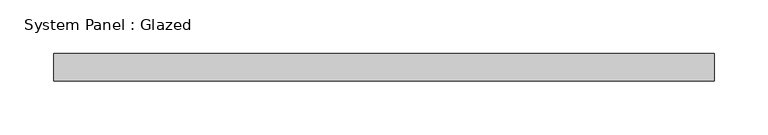
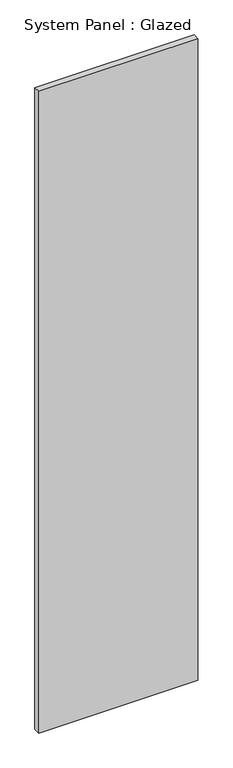
"""IFC4 building model written with IfcOpenShell, lengths in millimetres: plate geometry, System Panel : Glazed."""

from ifc_helpers import new_model, si_unit, origin, origin_with_axes, place, context, project, spatial, polyline, outline, extrude, source, transform, mapped, element, save


def system_panel_glazed_f1f14fe1(model_context):
    return source(origin(), model_context, "Body", "SweptSolid", [
        extrude(outline(polyline([(306.9166667, 19.05), (-306.9166667, 19.05), (-306.9166667, 44.45), (306.9166667, 44.45), (306.9166667, 19.05)])), origin_with_axes(), (0.0, 0.0, 1.0), 2616.2),
    ])


if __name__ == "__main__":
    model = new_model("IFC4")
    model_context = context("Model", 3, world=origin())
    ifc_project = project(units=[si_unit("LENGTHUNIT", "METRE", prefix="MILLI")], contexts=[model_context])
    site = spatial("IfcSite", under=ifc_project)
    building = spatial("IfcBuilding", under=site)
    placement = place(None, origin())
    system_panel_glazed_shape = system_panel_glazed_f1f14fe1(model_context)
    element("IfcPlate", 1, ObjectType="System Panel : Glazed", at=placement, inside=building, context=model_context, shape_type="MappedRepresentation", body=[
        mapped(system_panel_glazed_shape, transform((0.0, 0.0, 0.0), x_axis=(1.0, 0.0, 0.0), y_axis=(0.0, 1.0, 0.0), z_axis=(0.0, 0.0, 1.0))),
    ])
    save(model, "model.ifc")

# Revit data of these elements
# Type "System Panel : Glazed"
#   Construction Type Id = "GSP4R"
#   Analytic Construction = "1/8 in Pilkington single glazing"
#   Visual Light Transmittance = 0.9
#   Solar Heat Gain Coefficient = 0.86
#   Heat Transfer Coefficient (U) = 1.18115 BTU/(h·ft²·°F)
#   Define Thermal Properties by = 1
# Element 1 (IfcPlate, "System Panel : Glazed")
#   Materials on its faces: "Glass"
# Materials
#   "Glass": class "Glass", colour RGB 0 128 192, transparency 0.75, Description = "Soda Lime Glass", Cost = 0
